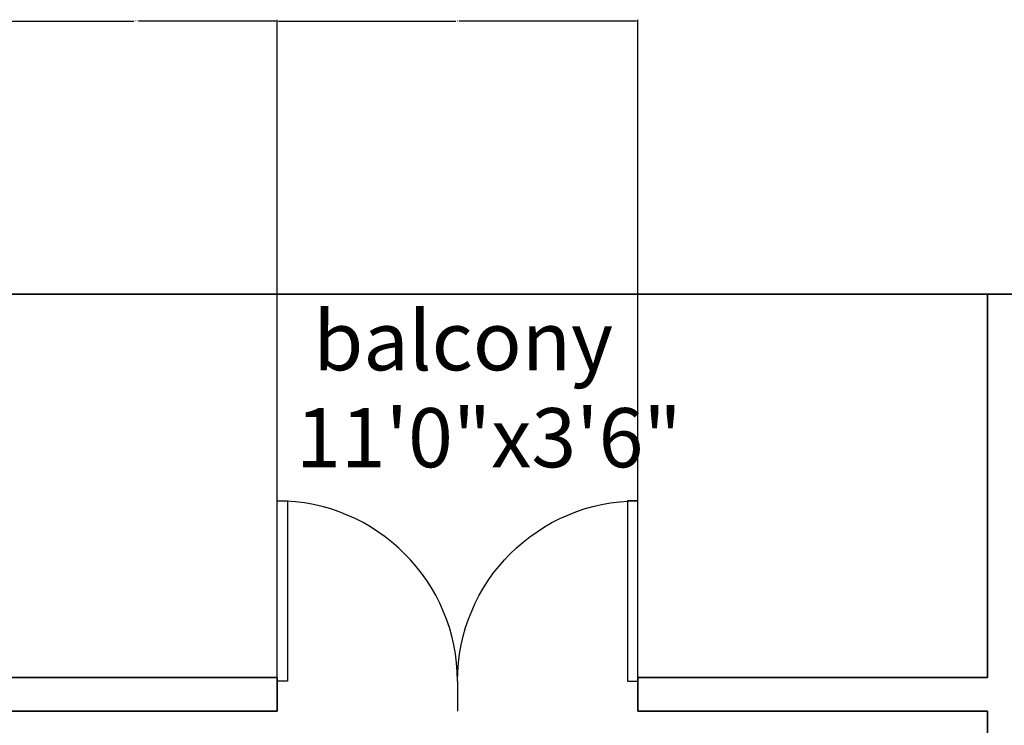
# Model space of a CAD drawing. Units: inches. Extents: x 108 to 613, y 1573 to 2319.
# Tile 10 of 11: x 303 to 434, y 2225 to 2319. Entities that reach past the tile are written whole.
import ezdxf

# ---------------------------------------------------------------- set-up
doc = ezdxf.new("R2010")
doc.units = ezdxf.units.IN
for name, color, linetype, lineweight in [('A-ANNO-DIMS', 2, 'Continuous', 18), ('A-AREA-IDEN', 3, 'Continuous', 18), ('door', 4, 'Continuous', 25), ('wall', 6, 'Continuous', 35)]:
    doc.layers.add(name, color=color, linetype=linetype, lineweight=lineweight)
doc.styles.get("Standard").update_dxf_attribs({"font": 'arial.ttf'})
doc.dimstyles.get("Standard").update_dxf_attribs({"dimtxt": 0.18, "dimasz": 0.18, "dimexe": 0.18, "dimexo": 0.0625, "dimgap": 0.09, "dimtad": 0, "dimtih": 1, "dimtoh": 1, "dimdec": 4, "dimzin": 0, "dimdsep": 46, "dimtxsty": 'Standard', "dimcen": 0.09, "dimadec": 0, "dimazin": 0, "dimtfac": 1, "dimtdec": 4, "dimtofl": 0, "dimtmove": 0, "dimatfit": 3, "dimfxl": 1, "dimtolj": 1, "dimtzin": 0, "dimarcsym": 0})

# ---------------------------------------------------------------- blocks, each defined once
blk = doc.blocks.new('*U2')
for p, q in [((0, 0), (0, -5)), ((30, 0), (30, -5))]:
    blk.add_line(p, q)
blk.add_lwpolyline([(0, 0), (0, 30), (1.75, 30), (1.75, 0)], close=True)
blk.add_arc((0, 0), 30, 0, 90)
blk = doc.blocks.new('*D46')
at = {"layer": 'A-ANNO-DIMS', "color": 0, "lineweight": -2, "transparency": 16777216}
for p, q in [((336.78, 2227.17), (336.78, 2319.14)), ((336.96, 2318.96), (360.55, 2318.96)), ((384.6, 2318.96), (361, 2318.96)), ((384.78, 2227.17), (384.78, 2319.14))]:
    blk.add_line(p, q, dxfattribs=at)
at = {"layer": 'A-ANNO-DIMS', "color": 0, "transparency": 16777216}
for points in [[(336.96, 2318.99), (336.96, 2318.93), (336.78, 2318.96)], [(384.6, 2318.99), (384.6, 2318.93), (384.78, 2318.96)]]:
    blk.add_solid(points, dxfattribs=at)
at = {"layer": 'Defpoints', "color": 0, "transparency": 16777216}
for p in [(384.78, 2318.96), (336.78, 2227.11), (384.78, 2227.11)]:
    blk.add_point(p, dxfattribs=at)
at = {"layer": 'A-ANNO-DIMS', "color": 0, "transparency": 16777216, "insert": (360.78, 2318.96), "char_height": 0.18, "attachment_point": 5}
blk.add_mtext('\\A1;48', dxfattribs=at)
blk = doc.blocks.new('*D47')
at = {"layer": 'A-ANNO-DIMS', "color": 0, "lineweight": -2, "transparency": 16777216}
for p, q in [((299.28, 2231.67), (299.28, 2319.14)), ((299.46, 2318.96), (317.7, 2318.96)), ((336.6, 2318.96), (318.35, 2318.96)), ((336.78, 2231.67), (336.78, 2319.14))]:
    blk.add_line(p, q, dxfattribs=at)
at = {"layer": 'A-ANNO-DIMS', "color": 0, "transparency": 16777216}
for points in [[(299.46, 2318.99), (299.46, 2318.93), (299.28, 2318.96)], [(336.6, 2318.99), (336.6, 2318.93), (336.78, 2318.96)]]:
    blk.add_solid(points, dxfattribs=at)
at = {"layer": 'Defpoints', "color": 0, "transparency": 16777216}
for p in [(336.78, 2318.96), (299.28, 2231.61), (336.78, 2231.61)]:
    blk.add_point(p, dxfattribs=at)
at = {"layer": 'A-ANNO-DIMS', "color": 0, "transparency": 16777216, "insert": (318.03, 2318.96), "char_height": 0.18, "attachment_point": 5}
blk.add_mtext('\\A1;37.5', dxfattribs=at)

msp = doc.modelspace()

# ---------------------------------------------------------------- linework, layer by layer
at = {"layer": 'wall'}
for p, q in [((294.7753, 2282.6125), (435.7753, 2282.6125)), ((431.2753, 2282.6125), (431.2753, 2231.6125)), ((299.2753, 2231.6125), (336.7753, 2231.6125)), ((336.7753, 2227.1125), (336.7753, 2231.6125)), ((384.7753, 2227.1125), (384.7753, 2231.6125)), ((384.7753, 2231.6125), (431.2753, 2231.6125)), ((299.2753, 2227.1125), (336.7753, 2227.1125)), ((384.7753, 2227.1125), (431.2753, 2227.1125)), ((431.2753, 2227.1125), (431.2753, 2134.1125))]:
    msp.add_line(p, q, dxfattribs=at)

# ---------------------------------------------------------------- block references
at = {"layer": 'door', "yscale": 0.8, "zscale": 0.8}
for p, xscale in [((336.7753, 2231.1125), 0.8), ((384.7753, 2231.1125), -0.8)]:
    msp.add_blockref('*U2', p, dxfattribs=dict(at, xscale=xscale))

# ---------------------------------------------------------------- texts
at = {"layer": 'A-AREA-IDEN'}
for s, p in [('balcony', (341.5999, 2272.4861)), ('11\'0"x3\'6"', (339.2916, 2259.5802))]:
    msp.add_text(s, height=7.87346, dxfattribs=at).set_placement(p)

# ---------------------------------------------------------------- dimensions: what is measured, and where the dimension line sits
at = {"layer": 'A-ANNO-DIMS'}
for base, p1, p2, override, picture, middle in [((336.7753, 2318.9625), (299.2753, 2231.6125), (336.7753, 2231.6125), {"dimdec": 1, "dimlfac": 1, "dimrnd": 0, "dimzin": 0, "dimdsep": 46, "dimlunit": 2}, '*D47', (318.0253, 2318.9625)), ((384.7753, 2318.9625), (336.7753, 2227.1125), (384.7753, 2227.1125), {"dimdec": 0, "dimlfac": 1, "dimrnd": 0, "dimzin": 0, "dimdsep": 46, "dimlunit": 2}, '*D46', (360.7753, 2318.9625))]:
    dim = msp.add_linear_dim(base=base, p1=p1, p2=p2, dimstyle='Standard', override=override, dxfattribs=at)
    dim.commit()
    dim.dimension.update_dxf_attribs({"geometry": picture, "text_midpoint": middle})

doc.saveas('drawing.dxf')
